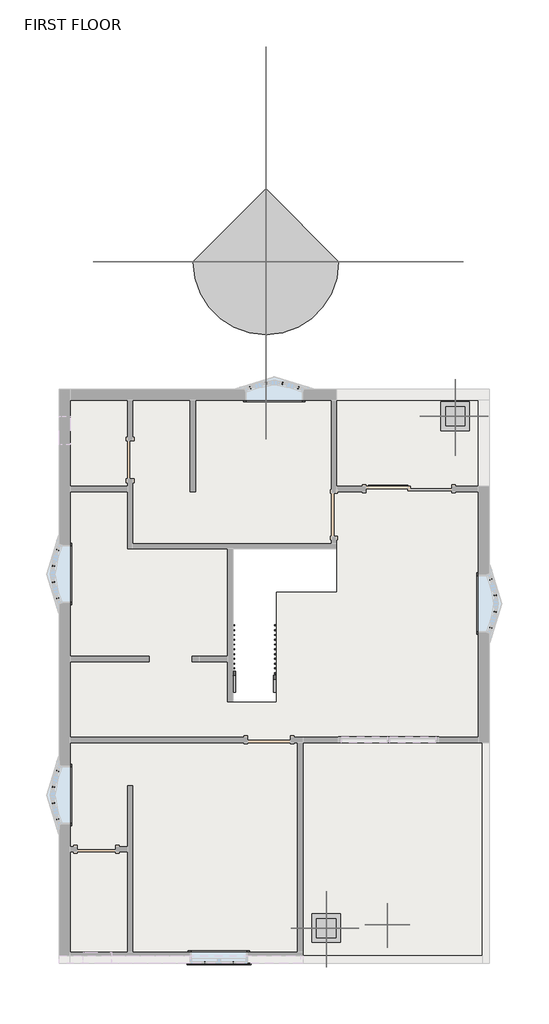
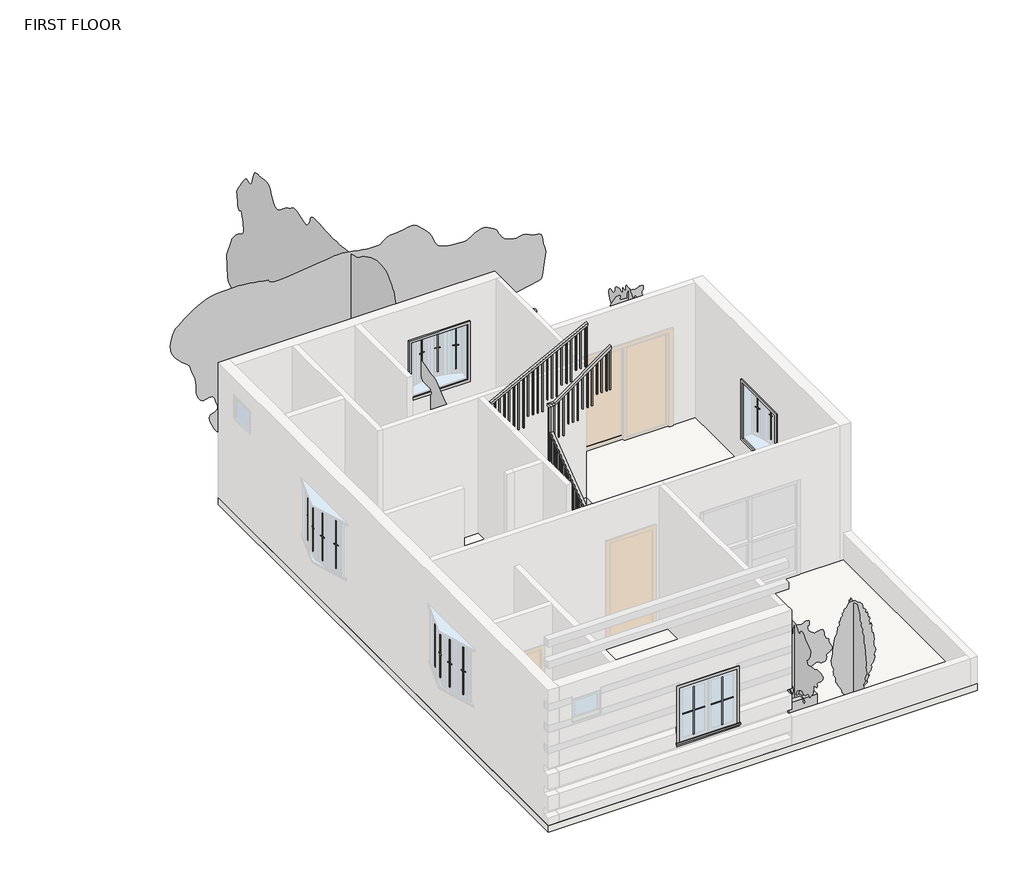
# One storey, part 2 of 2: 24 proxies, 6 geographic elements, 2 railings, 1 slab.
# Revit data of these elements (continued)
# Type "RPC Tree - Deciduous : Japanese Cherry - 15'" (continued)
#   built-in parameter 1005198 = "{2, 15},{39, RPC-16-FXGW-2MQ0-PN7K-A000-ST1L-LVER-AU},{1, 0},{1, 0},{2, 35},{1, 8},{5, Color},{1, 0},{1, 0},{3, 0.8},{3, 0.8},{3, 0.8},{1, 8},{7, BBoxMin},{1, 0},{1, 0},{1, 0},{1, 0},{1, 0},{1, 8},{7, BBoxMax},{1, 0},{1, 0},{1, 0},{1, 0},{1, 0},{2, 11},{9, RPCTypeId},{1, 0},{1, 0},{39, RPC-16-FXGW-2MQ0-PN7K-A000-ST1L-LVER-AU},{1, 6},{14, RPCPlantHeight},{1, 0},{1, 0},{2, 15},{2, 11},{7, keyword},{1, 0},{1, 0},{207, :Geometry:RPC:Japanese Flowering Cherry:Prunus serrulata Lindl:A landscape tree:valued for its abundant showy flowers; native to China and Japan.  Hardy only in the mildest parts of Canada and farther south.},{2, 11},{8, category},{1, 0},{1, 0},{16, :Trees [General]},{2, 11},{12, LocalizedUID},{1, 0},{1, 0},{25, Japanese Flowering Cherry},{2, 14},{6, Height},{1, 0},{1, 0},{2, 15},{1, 2},{16, Cast Reflections},{1, 0},{1, 0},{1, 0},{1, 2},{12, Cast Shadows},{1, 0},{1, 0},{1, 1},{1, 2},{9, Lock View},{1, 0},{1, 0},{1, 0},{1, 4},{5, ViewC},{1, 0},{1, 0},{1, 0},{2, 11},{20, AdvancedUIDefinition},{1, 0},{1, 0},{0, },{2, 11},{10, AssetLibID},{1, 0},{1, 0},{36, 4D3F6E72-3F99-4203-98E9-AF80B3C7A7A4},{2, 11},{10, BaseSchema},{1, 0},{1, 0},{9, RPCSchema},{2, 11},{12, ExchangeGUID},{1, 0},{1, 0},{0, },{1, 2},{6, Hidden},{1, 0},{1, 0},{1, 0},{1, 4},{11, RPCCategory},{1, 0},{1, 0},{1, 0},{2, 11},{8, RPCImage},{1, 0},{1, 0},{0, },{1, 4},{13, SchemaVersion},{1, 0},{1, 0},{1, 4},{2, 11},{12, UIDefinition},{1, 0},{1, 0},{0, },{2, 11},{6, UIName},{1, 0},{1, 0},{39, RPC-16-FXGW-2MQ0-PN7K-A000-ST1L-LVER-AU},{2, 11},{11, VersionGUID},{1, 0},{1, 0},{9, RPCSchema},{2, 11},{9, assettype},{1, 0},{1, 0},{11, RPCGeometry},{2, 11},{11, description},{1, 0},{1, 0},{0, },{2, 11},{9, localname},{1, 0},{1, 0},{3, RPC},{2, 11},{9, localtype},{1, 0},{1, 0},{3, RPC},{1, 4},{8, revision},{1, 0},{1, 0},{1, 1},{2, 11},{9, thumbnail},{1, 0},{1, 0},{0, },{1, 4},{7, version},{1, 0},{1, 0},{1, 1},{1, 2},{20, RPC_Cast Reflections},{1, 0},{1, 0},{1, 1},{1, 2},{16, RPC_Cast Shadows},{1, 0},{1, 0},{1, 1},{1, 2},{13, RPC_Lock View},{1, 0},{1, 0},{1, 0},{1, 4},{9, RPC_ViewC},{1, 0},{1, 0},{1, 0},{21, assetlibrary_base.fbx},{1, 5},"
#   built-in parameter 1005195 = "RPC-16-FXGW-2MQ0-PN7K-A000-ST1L-LVER-AU"
#   Type Comments = "Japanese Cherry"
#   Assembly Code = "G2050500"
#   Height = 7' - 0"
#   Default Elevation = 0
# Type "Handrail - Rectangular"
#   Assembly Code = "C2010400"
#   built-in parameter 1008612 = 0.0416667 (stored number, unit not read)
#   built-in parameter 1008611 = 0.0416667 (stored number, unit not read)
#   built-in parameter 1008609 = 0.333333 (stored number, unit not read)
#   built-in parameter 1008604 = 0.166667 (stored number, unit not read)
#   built-in parameter 1008603 = 0.166667 (stored number, unit not read)
#   Railing Height = 2' - 6"
#   built-in parameter 1008630 = 2
#   built-in parameter 1008610 = 2
#   built-in parameter 1008618 = Baluster - Square : 3/4"
# Type "6\""
#   Assembly Code = "B1010"
#   Function = 0
#   Layers, outside or top first: 0' - 6" no material (function 1)
# Elements 1, 2, 3, 4, 5, 6, 7, 8, 9, 10, 11, 12, 13, 14, 15, 16 (IfcBuildingElementProxy, "Muntin Pattern_2x2 : Muntin Pattern_2x2")
#   Width = 0' - 4.43605"
#   Height = 3' - 6 1/2"
#   Interior Material = Wood - Stained
#   Exterior Material = Clad - White
#   Phase Created = New Construction
#   Materials on its faces: "Clad - White", "Wood - Stained"
# Elements 17, 18 (IfcBuildingElementProxy, "Muntin Pattern_2x2 : Muntin Pattern_2x2")
#   Width = 1' - 6 5/8"
#   Height = 3' - 6 1/2"
#   Interior Material = Wood - Stained
#   Exterior Material = Clad - White
#   Phase Created = New Construction
#   Materials on its faces: "Clad - White", "Wood - Stained"
# Element 19 (IfcBuildingElementProxy, "Trim-Window-Exterior-Flat : with Sill")
#   Opening Width = 4' - 0"
#   Opening Height = 4' - 0"
#   Trim Material = Clad - White
#   Phase Created = New Construction
#   Materials on its faces: "Clad - White"
# Elements 20, 21, 22, 23 (IfcBuildingElementProxy, "Trim-Window-Interior-Flat : Picture Frame")
#   Opening Width = 4' - 0"
#   Opening Height = 4' - 2"
#   Trim Material = Wood - Stained
#   Phase Created = New Construction
#   Materials on its faces: "Wood - Stained"
# Element 24 (IfcBuildingElementProxy, "Trim-Window-Interior-Flat : Picture Frame")
#   Opening Width = 4' - 0"
#   Opening Height = 4' - 0"
#   Trim Material = Wood - Stained
#   Phase Created = New Construction
#   Materials on its faces: "Wood - Stained"
# Elements 25, 26 (IfcGeographicElement, "Planter : 2'x2'")
#   Phase Created = New Construction
#   Materials on its faces: "Concrete, Precast"
# Element 27 (IfcGeographicElement, "RPC Tree - Conifer : Chinese Juniper - 7'")
#   Phase Created = New Construction
# Element 28 (IfcGeographicElement, "RPC Tree - Deciduous : Common Apple - 20' 2")
#   Phase Created = New Construction
# Elements 29, 30 (IfcGeographicElement, "RPC Tree - Deciduous : Japanese Cherry - 15'")
#   Phase Created = New Construction
# Elements 31, 32 (IfcRailing, "Handrail - Rectangular")
#   Phase Created = New Construction
# Element 33 (IfcSlab, "6\"")
#   Height Offset From Level = 0' - 0"
#   Phase Created = New Construction
#   Materials on its faces: "Default Floor", "wall 1", "6\" wall"
# Materials
#   "Concrete, Precast": class "Concrete", colour RGB 198 187 187, transparency 0, Description = "Precast concrete", Cost = 0
#   "Clad - White": class "Wood", colour RGB 242 242 238, transparency 0, Cost = 0
#   "Wood - Stained": class "Wood", colour RGB 224 178 126, transparency 0, Cost = 0
#   "Default Floor": colour RGB 128 128 128, transparency 0, Cost = 0
#   "wall 1": class "Generic", colour RGB 67 39 34, transparency 0, Cost = 0
#   "6\" wall": class "Generic", colour RGB 177 162 144, transparency 0, Cost = 0
